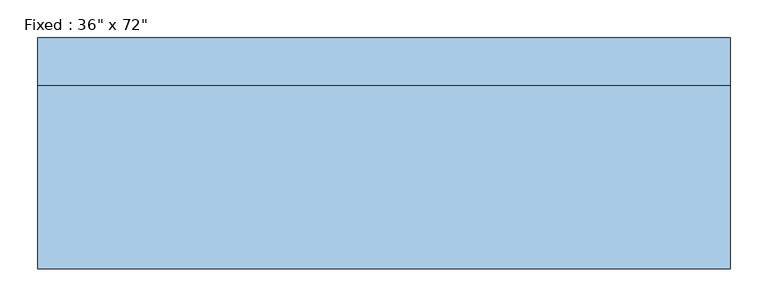
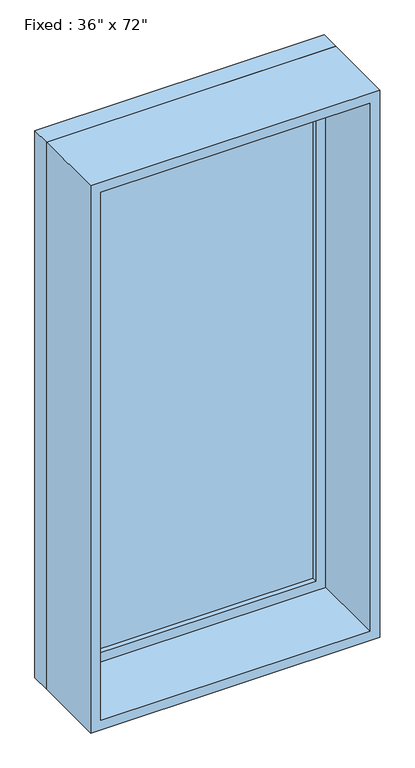
"""IFC4 building model written with IfcOpenShell, lengths in millimetres: window geometry."""

from ifc_helpers import new_model, si_unit, frame, origin, place, context, project, spatial, polyline, outline, extrude, source, transform, mapped, element, save


def window_c524ad49(model_context):
    return source(origin(), model_context, "Body", "SweptSolid", [
        extrude(outline(polyline([(355.6, 104.775), (-431.8, 104.775), (-431.8, 117.475), (355.6, 117.475), (355.6, 104.775)])), frame((0.0, 0.0, 368.3), z_axis=(0.0, 0.0, 1.0), x_axis=(1.0, 0.0, 0.0)), (0.0, 0.0, 1.0), 1701.8),
        extrude(outline(polyline([(2114.55, -476.25), (323.85, -476.25), (323.85, 400.05), (2114.55, 400.05), (2114.55, -476.25)]), holes=[polyline([(2070.1, -431.8), (2070.1, 355.6), (368.3, 355.6), (368.3, -431.8), (2070.1, -431.8)])]), frame((0.0, 88.9, 0.0), z_axis=(0.0, 1.0, 0.0), x_axis=(0.0, 0.0, 1.0)), (0.0, 0.0, 1.0), 44.45),
        extrude(outline(polyline([(2133.6, -495.3), (304.8, -495.3), (304.8, 419.1), (2133.6, 419.1), (2133.6, -495.3)]), holes=[polyline([(2101.85, -463.55), (2101.85, 387.35), (336.55, 387.35), (336.55, -463.55), (2101.85, -463.55)])]), frame((0.0, -152.4, 0.0), z_axis=(0.0, 1.0, 0.0), x_axis=(0.0, 0.0, 1.0)), (0.0, 0.0, 1.0), 241.3),
        extrude(outline(polyline([(2133.6, 419.1), (2133.6, -495.3), (304.8, -495.3), (304.8, 419.1), (2133.6, 419.1)]), holes=[polyline([(2114.55, 400.05), (323.85, 400.05), (323.85, -476.25), (2114.55, -476.25), (2114.55, 400.05)])]), frame((0.0, 88.9, 0.0), z_axis=(0.0, 1.0, 0.0), x_axis=(0.0, 0.0, 1.0)), (0.0, 0.0, 1.0), 63.5),
    ])


if __name__ == "__main__":
    model = new_model("IFC4")
    model_context = context("Model", 3, world=origin())
    ifc_project = project(units=[si_unit("LENGTHUNIT", "METRE", prefix="MILLI")], contexts=[model_context])
    site = spatial("IfcSite", under=ifc_project)
    building = spatial("IfcBuilding", under=site)
    placement = place(None, origin())
    window_shape = window_c524ad49(model_context)
    element("IfcWindow", 1, ObjectType="Fixed : 36\" x 72\"", at=placement, inside=building, context=model_context, shape_type="MappedRepresentation", body=[
        mapped(window_shape, transform((0.0, 0.0, 0.0), x_axis=(1.0, 0.0, 0.0), y_axis=(0.0, 1.0, 0.0), z_axis=(0.0, 0.0, 1.0))),
    ])
    save(model, "model.ifc")

# Revit data of these elements
# Type "Fixed : 36\" x 72\""
#   Type Mark = "9"
#   Construction Type Id = "GSP4R"
#   Assembly Code = "B2020100"
#   Analytic Construction = "1/8 in Pilkington single glazing"
#   Visual Light Transmittance = 0.9
#   Solar Heat Gain Coefficient = 0.78
#   Heat Transfer Coefficient (U) = 0.6496 BTU/(h·ft²·°F)
#   Height = 6' - 0"
#   Default Sill Height = 1' - 0"
#   Width = 3' - 0"
#   Window Inset = 0' - 0 3/4"
#   Define Thermal Properties by = 1
#   Glass Pane Material = Glass
#   Sash Material = Iron, Ductile
#   Wall Closure = (empty or 0)
# Element 1 (IfcWindow, "Fixed : 36\" x 72\"")
#   Materials on its faces: "Iron, Ductile", "Glass"
# Materials
#   "Glass": class "Glass", colour RGB 0 128 192, transparency 0.75, Description = "Soda Lime Glass", Cost = 0
#   "Iron, Ductile": class "Metal", colour RGB 0 0 0, transparency 0, Description = "Ductile cast iron", Cost = 0
